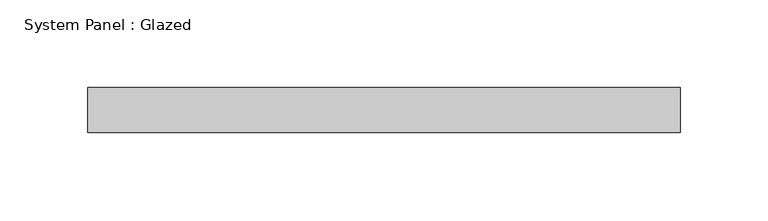
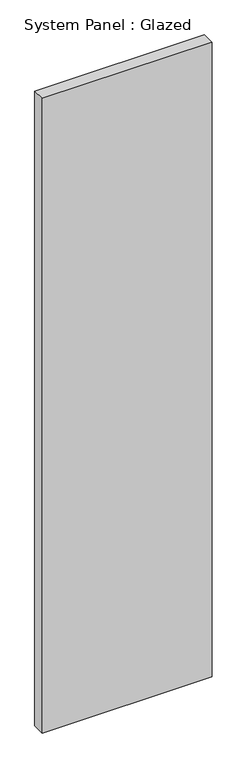
"""IFC4 building model written with IfcOpenShell, lengths in millimetres: plate geometry, System Panel : Glazed."""

from ifc_helpers import new_model, si_unit, origin, origin_with_axes, place, context, project, spatial, polyline, outline, extrude, source, transform, mapped, element, save


def system_panel_glazed_e40eab22(model_context):
    return source(origin(), model_context, "Body", "SweptSolid", [
        extrude(outline(polyline([(168.275, 19.05), (-168.275, 19.05), (-168.275, 44.45), (168.275, 44.45), (168.275, 19.05)])), origin_with_axes(), (0.0, 0.0, 1.0), 1329.6512079),
    ])


if __name__ == "__main__":
    model = new_model("IFC4")
    model_context = context("Model", 3, world=origin())
    ifc_project = project(units=[si_unit("LENGTHUNIT", "METRE", prefix="MILLI")], contexts=[model_context])
    site = spatial("IfcSite", under=ifc_project)
    building = spatial("IfcBuilding", under=site)
    placement = place(None, origin())
    system_panel_glazed_shape = system_panel_glazed_e40eab22(model_context)
    element("IfcPlate", 1, ObjectType="System Panel : Glazed", at=placement, inside=building, context=model_context, shape_type="MappedRepresentation", body=[
        mapped(system_panel_glazed_shape, transform((0.0, 0.0, 0.0), x_axis=(1.0, 0.0, 0.0), y_axis=(0.0, 1.0, 0.0), z_axis=(0.0, 0.0, 1.0))),
    ])
    save(model, "model.ifc")

# Revit data of these elements
# Type "System Panel : Glazed"
#   Construction Type Id = "GSP4R"
#   Analytic Construction = "1/8 in Pilkington single glazing"
#   Visual Light Transmittance = 0.9
#   Solar Heat Gain Coefficient = 0.86
#   Heat Transfer Coefficient (U) = 1.18115 BTU/(h·ft²·°F)
#   Define Thermal Properties by = 1
# Element 1 (IfcPlate, "System Panel : Glazed")
#   Materials on its faces: "Glass"
# Materials
#   "Glass": class "Glass", colour RGB 0 128 192, transparency 0.75, Description = "Soda Lime Glass", Cost = 0
